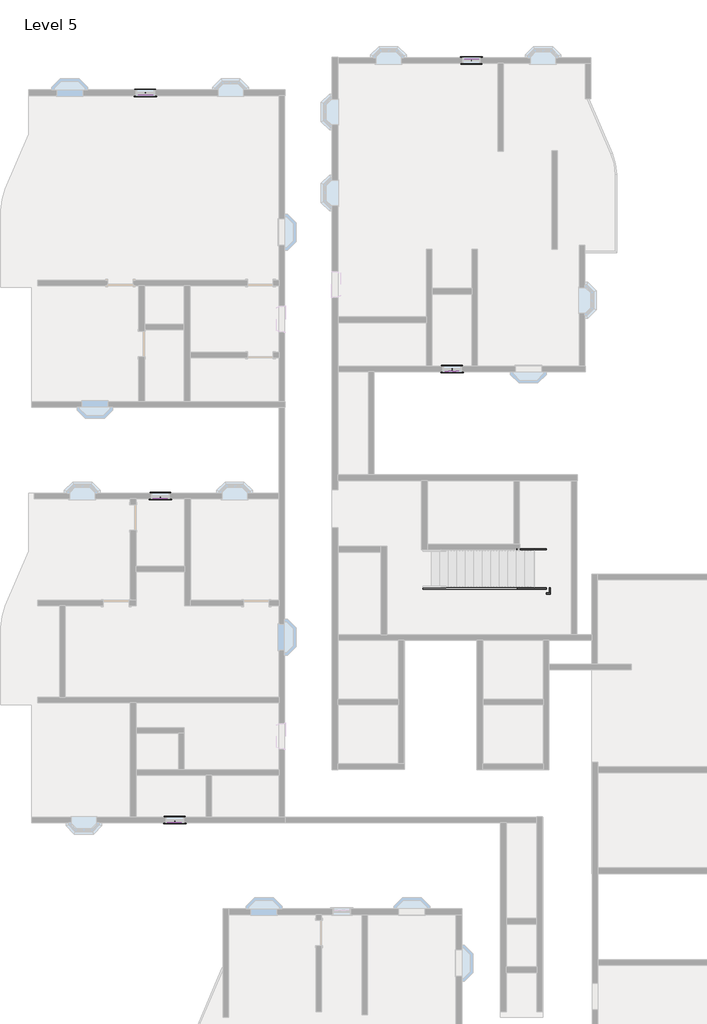
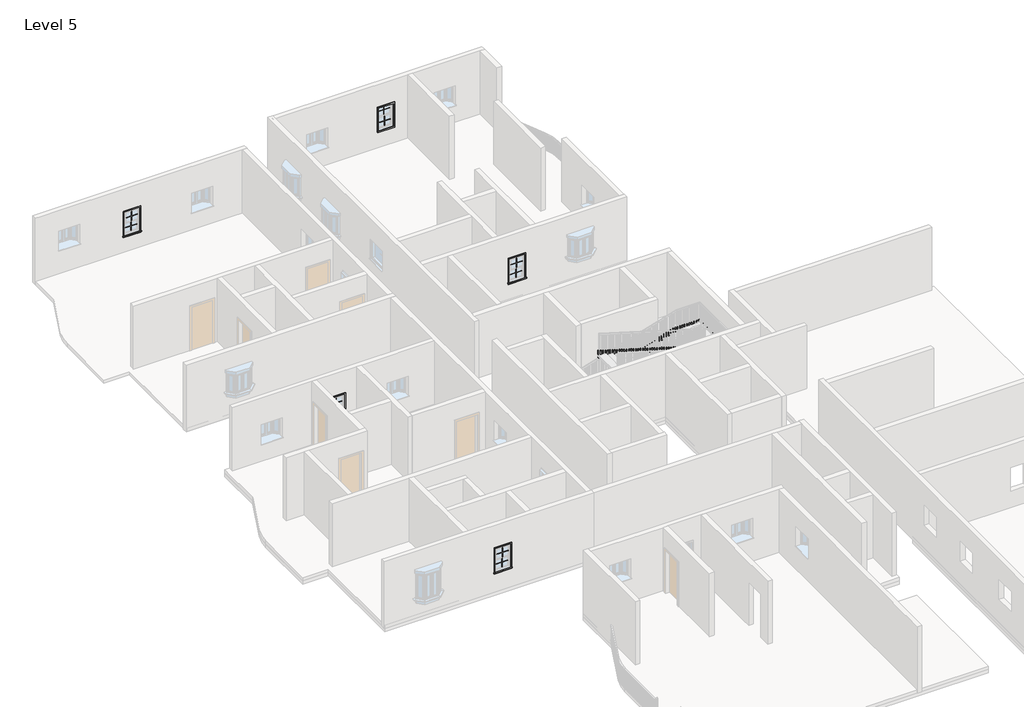
# One storey, part 14 of 14: 20 proxies, 6 members.
"""IFC4 building model written with IfcOpenShell, lengths in millimetres."""

from ifc_helpers import new_model, si_unit, frame, origin, place, context, project, spatial, polyline, outline, extrude, transform, mapped, element, save
from components import muntin_pattern_2x2_muntin_pattern_2x2_c35c595f, trim_window_exterior_flat_with_sill_e38017c9, trim_window_interior_flat_picture_frame_d728ed12

model = new_model("IFC4")

# Units and contexts
model_context = context("Model", 3, world=origin())
ifc_project = project(units=[si_unit("LENGTHUNIT", "METRE", prefix="MILLI")], contexts=[model_context])

# Site, building, storey
site = spatial("IfcSite", under=ifc_project)
building = spatial("IfcBuilding", under=site)
storey = spatial("IfcBuildingStorey", under=building, Name="Level 5", Elevation=12192.0)

# Proxies
placement = place(None, origin())
muntin_pattern_2x2_muntin_pattern_2x2_shape = muntin_pattern_2x2_muntin_pattern_2x2_c35c595f(model_context)
element("IfcBuildingElementProxy", 1, Name="Muntin Pattern_2x2 : Muntin Pattern_2x2", ObjectType="Muntin Pattern_2x2 : Muntin Pattern_2x2", at=placement, inside=storey, context=model_context, shape_type="MappedRepresentation", body=[
    mapped(muntin_pattern_2x2_muntin_pattern_2x2_shape, transform((-14639.3891351, 14368.0833494, 13662.025), x_axis=(-1.0, 0.0, 0.0), y_axis=(0.0, -1.0, 0.0), z_axis=(0.0, 0.0, 1.0))),
])
element("IfcBuildingElementProxy", 2, Name="Muntin Pattern_2x2 : Muntin Pattern_2x2", ObjectType="Muntin Pattern_2x2 : Muntin Pattern_2x2", at=placement, inside=storey, context=model_context, shape_type="MappedRepresentation", body=[
    mapped(muntin_pattern_2x2_muntin_pattern_2x2_shape, transform((-14639.3891351, 14412.5333494, 13182.6), x_axis=(-1.0, 0.0, 0.0), y_axis=(0.0, -1.0, 0.0), z_axis=(0.0, 0.0, 1.0))),
])
element("IfcBuildingElementProxy", 3, Name="Muntin Pattern_2x2 : Muntin Pattern_2x2", ObjectType="Muntin Pattern_2x2 : Muntin Pattern_2x2", at=placement, inside=storey, context=model_context, shape_type="MappedRepresentation", body=[
    mapped(muntin_pattern_2x2_muntin_pattern_2x2_shape, transform((-14125.0391351, 2785.6833494, 13662.025), x_axis=(-1.0, 0.0, 0.0), y_axis=(0.0, -1.0, 0.0), z_axis=(0.0, 0.0, 1.0))),
])
element("IfcBuildingElementProxy", 4, Name="Muntin Pattern_2x2 : Muntin Pattern_2x2", ObjectType="Muntin Pattern_2x2 : Muntin Pattern_2x2", at=placement, inside=storey, context=model_context, shape_type="MappedRepresentation", body=[
    mapped(muntin_pattern_2x2_muntin_pattern_2x2_shape, transform((-14125.0391351, 2830.1333494, 13182.6), x_axis=(-1.0, 0.0, 0.0), y_axis=(0.0, -1.0, 0.0), z_axis=(0.0, 0.0, 1.0))),
])
element("IfcBuildingElementProxy", 5, Name="Muntin Pattern_2x2 : Muntin Pattern_2x2", ObjectType="Muntin Pattern_2x2 : Muntin Pattern_2x2", at=placement, inside=storey, context=model_context, shape_type="MappedRepresentation", body=[
    mapped(muntin_pattern_2x2_muntin_pattern_2x2_shape, transform((-4206.3391351, 18910.0465905, 13662.025), x_axis=(-1.0, 0.0, 0.0), y_axis=(0.0, -1.0, 0.0), z_axis=(0.0, 0.0, 1.0))),
])
element("IfcBuildingElementProxy", 6, Name="Muntin Pattern_2x2 : Muntin Pattern_2x2", ObjectType="Muntin Pattern_2x2 : Muntin Pattern_2x2", at=placement, inside=storey, context=model_context, shape_type="MappedRepresentation", body=[
    mapped(muntin_pattern_2x2_muntin_pattern_2x2_shape, transform((-4206.3391351, 18954.4965905, 13182.6), x_axis=(-1.0, 0.0, 0.0), y_axis=(0.0, -1.0, 0.0), z_axis=(0.0, 0.0, 1.0))),
])
element("IfcBuildingElementProxy", 7, Name="Muntin Pattern_2x2 : Muntin Pattern_2x2", ObjectType="Muntin Pattern_2x2 : Muntin Pattern_2x2", at=placement, inside=storey, context=model_context, shape_type="MappedRepresentation", body=[
    mapped(muntin_pattern_2x2_muntin_pattern_2x2_shape, transform((-3514.1891351, 30066.9965905, 13662.025), x_axis=(1.0, 0.0, 0.0), y_axis=(0.0, 1.0, 0.0), z_axis=(0.0, 0.0, 1.0))),
])
element("IfcBuildingElementProxy", 8, Name="Muntin Pattern_2x2 : Muntin Pattern_2x2", ObjectType="Muntin Pattern_2x2 : Muntin Pattern_2x2", at=placement, inside=storey, context=model_context, shape_type="MappedRepresentation", body=[
    mapped(muntin_pattern_2x2_muntin_pattern_2x2_shape, transform((-3514.1891351, 30022.5465905, 13182.6), x_axis=(1.0, 0.0, 0.0), y_axis=(0.0, 1.0, 0.0), z_axis=(0.0, 0.0, 1.0))),
])
element("IfcBuildingElementProxy", 9, Name="Muntin Pattern_2x2 : Muntin Pattern_2x2", ObjectType="Muntin Pattern_2x2 : Muntin Pattern_2x2", at=placement, inside=storey, context=model_context, shape_type="MappedRepresentation", body=[
    mapped(muntin_pattern_2x2_muntin_pattern_2x2_shape, transform((-15175.9641351, 28782.5833494, 13662.025), x_axis=(-1.0, 0.0, 0.0), y_axis=(0.0, -1.0, 0.0), z_axis=(0.0, 0.0, 1.0))),
])
element("IfcBuildingElementProxy", 10, Name="Muntin Pattern_2x2 : Muntin Pattern_2x2", ObjectType="Muntin Pattern_2x2 : Muntin Pattern_2x2", at=placement, inside=storey, context=model_context, shape_type="MappedRepresentation", body=[
    mapped(muntin_pattern_2x2_muntin_pattern_2x2_shape, transform((-15175.9641351, 28827.0333494, 13182.6), x_axis=(-1.0, 0.0, 0.0), y_axis=(0.0, -1.0, 0.0), z_axis=(0.0, 0.0, 1.0))),
])
trim_window_exterior_flat_with_sill_shape = trim_window_exterior_flat_with_sill_e38017c9(model_context)
element("IfcBuildingElementProxy", 11, Name="Trim-Window-Exterior-Flat : with Sill", ObjectType="Trim-Window-Exterior-Flat : with Sill", at=placement, inside=storey, context=model_context, shape_type="MappedRepresentation", body=[
    mapped(trim_window_exterior_flat_with_sill_shape, transform((-14639.3891351, 14333.1583494, 14173.2), x_axis=(1.0, 0.0, 0.0), y_axis=(0.0, 0.0, 1.0), z_axis=(0.0, -1.0, 0.0))),
])
element("IfcBuildingElementProxy", 12, Name="Trim-Window-Exterior-Flat : with Sill", ObjectType="Trim-Window-Exterior-Flat : with Sill", at=placement, inside=storey, context=model_context, shape_type="MappedRepresentation", body=[
    mapped(trim_window_exterior_flat_with_sill_shape, transform((-14125.0391351, 2750.7583494, 14173.2), x_axis=(1.0, 0.0, 0.0), y_axis=(0.0, 0.0, 1.0), z_axis=(0.0, -1.0, 0.0))),
])
element("IfcBuildingElementProxy", 13, Name="Trim-Window-Exterior-Flat : with Sill", ObjectType="Trim-Window-Exterior-Flat : with Sill", at=placement, inside=storey, context=model_context, shape_type="MappedRepresentation", body=[
    mapped(trim_window_exterior_flat_with_sill_shape, transform((-4206.3391351, 18875.1215905, 14173.2), x_axis=(1.0, 0.0, 0.0), y_axis=(0.0, 0.0, 1.0), z_axis=(0.0, -1.0, 0.0))),
])
element("IfcBuildingElementProxy", 14, Name="Trim-Window-Exterior-Flat : with Sill", ObjectType="Trim-Window-Exterior-Flat : with Sill", at=placement, inside=storey, context=model_context, shape_type="MappedRepresentation", body=[
    mapped(trim_window_exterior_flat_with_sill_shape, transform((-3514.1891351, 30101.9215905, 14173.2), x_axis=(-1.0, 0.0, 0.0), y_axis=(0.0, 0.0, 1.0), z_axis=(0.0, 1.0, 0.0))),
])
element("IfcBuildingElementProxy", 15, Name="Trim-Window-Exterior-Flat : with Sill", ObjectType="Trim-Window-Exterior-Flat : with Sill", at=placement, inside=storey, context=model_context, shape_type="MappedRepresentation", body=[
    mapped(trim_window_exterior_flat_with_sill_shape, transform((-15175.9641351, 28747.6583494, 14173.2), x_axis=(1.0, 0.0, 0.0), y_axis=(0.0, 0.0, 1.0), z_axis=(0.0, -1.0, 0.0))),
])
trim_window_interior_flat_picture_frame_shape = trim_window_interior_flat_picture_frame_d728ed12(model_context)
element("IfcBuildingElementProxy", 16, Name="Trim-Window-Interior-Flat : Picture Frame", ObjectType="Trim-Window-Interior-Flat : Picture Frame", at=placement, inside=storey, context=model_context, shape_type="MappedRepresentation", body=[
    mapped(trim_window_interior_flat_picture_frame_shape, transform((-14639.3891351, 14536.3583494, 14173.2), x_axis=(-1.0, 0.0, 0.0), y_axis=(0.0, 0.0, 1.0), z_axis=(0.0, 1.0, 0.0))),
])
element("IfcBuildingElementProxy", 17, Name="Trim-Window-Interior-Flat : Picture Frame", ObjectType="Trim-Window-Interior-Flat : Picture Frame", at=placement, inside=storey, context=model_context, shape_type="MappedRepresentation", body=[
    mapped(trim_window_interior_flat_picture_frame_shape, transform((-14125.0391351, 2953.9583494, 14173.2), x_axis=(-1.0, 0.0, 0.0), y_axis=(0.0, 0.0, 1.0), z_axis=(0.0, 1.0, 0.0))),
])
element("IfcBuildingElementProxy", 18, Name="Trim-Window-Interior-Flat : Picture Frame", ObjectType="Trim-Window-Interior-Flat : Picture Frame", at=placement, inside=storey, context=model_context, shape_type="MappedRepresentation", body=[
    mapped(trim_window_interior_flat_picture_frame_shape, transform((-4206.3391351, 19078.3215905, 14173.2), x_axis=(-1.0, 0.0, 0.0), y_axis=(0.0, 0.0, 1.0), z_axis=(0.0, 1.0, 0.0))),
])
element("IfcBuildingElementProxy", 19, Name="Trim-Window-Interior-Flat : Picture Frame", ObjectType="Trim-Window-Interior-Flat : Picture Frame", at=placement, inside=storey, context=model_context, shape_type="MappedRepresentation", body=[
    mapped(trim_window_interior_flat_picture_frame_shape, transform((-3514.1891351, 29898.7215905, 14173.2), x_axis=(1.0, 0.0, 0.0), y_axis=(0.0, 0.0, 1.0), z_axis=(0.0, -1.0, 0.0))),
])
element("IfcBuildingElementProxy", 20, Name="Trim-Window-Interior-Flat : Picture Frame", ObjectType="Trim-Window-Interior-Flat : Picture Frame", at=placement, inside=storey, context=model_context, shape_type="MappedRepresentation", body=[
    mapped(trim_window_interior_flat_picture_frame_shape, transform((-15175.9641351, 28950.8583494, 14173.2), x_axis=(-1.0, 0.0, 0.0), y_axis=(0.0, 0.0, 1.0), z_axis=(0.0, 1.0, 0.0))),
])

# Members
element("IfcMember", 21, ObjectType="Stringer - 2\" Width", at=placement, inside=storey, context=model_context, shape_type="SweptSolid", body=[
    extrude(outline(polyline([(12383.5995961, -5254.0891351), (12192.0, -5254.0891351), (12192.0, -4832.019314), (13639.8, -6.019314), (13639.8, -1066.7544553), (12383.5995961, -5254.0891351)])), frame((0.0, 12506.0715905, 0.0), z_axis=(0.0, 1.0, 0.0), x_axis=(0.0, 0.0, 1.0)), (0.0, 0.0, 1.0), 50.8),
])
element("IfcMember", 22, ObjectType="Stringer - 2\" Width", at=placement, inside=storey, context=model_context, shape_type="SweptSolid", body=[
    extrude(outline(polyline([(54.5108649, 12556.8715905), (105.3108649, 12556.8715905), (105.3108649, 9478.4949943), (54.5108649, 9478.4949943), (54.5108649, 12556.8715905)])), frame((0.0, 0.0, 13335.0), z_axis=(0.0, 0.0, 1.0), x_axis=(1.0, 0.0, 0.0)), (0.0, 0.0, 1.0), 304.8),
])
element("IfcMember", 23, ObjectType="Stringer - 2\" Width", at=placement, inside=storey, context=model_context, shape_type="SweptSolid", body=[
    extrude(outline(polyline([(13335.0, 105.3108649), (13427.5395961, 105.3108649), (15035.3595961, -5254.0891351), (14717.1390537, -5254.0891351), (13335.0, -646.9589562), (13335.0, 105.3108649)])), frame((0.0, 9427.6949943, 0.0), z_axis=(0.0, 1.0, 0.0), x_axis=(0.0, 0.0, 1.0)), (0.0, 0.0, 1.0), 50.8),
])
element("IfcMember", 24, ObjectType="Stringer - 2\" Width", at=placement, inside=storey, context=model_context, shape_type="SweptSolid", body=[
    extrude(outline(polyline([(12383.5995961, -5254.0891351), (12192.0, -5254.0891351), (12192.0, -4832.019314), (13421.7390537, -732.8891351), (13639.8, -732.8891351), (13639.8, -1066.7544553), (12383.5995961, -5254.0891351)])), frame((0.0, 11103.4082924, 0.0), z_axis=(0.0, 1.0, 0.0), x_axis=(0.0, 0.0, 1.0)), (0.0, 0.0, 1.0), 50.8),
])
element("IfcMember", 25, ObjectType="Stringer - 2\" Width", at=placement, inside=storey, context=model_context, shape_type="SweptSolid", body=[
    extrude(outline(polyline([(-732.8891351, 11154.2082924), (-682.0891351, 11154.2082924), (-682.0891351, 10976.4082924), (-732.8891351, 10976.4082924), (-732.8891351, 11154.2082924)])), frame((0.0, 0.0, 13335.0), z_axis=(0.0, 0.0, 1.0), x_axis=(1.0, 0.0, 0.0)), (0.0, 0.0, 1.0), 304.8),
])
element("IfcMember", 26, ObjectType="Stringer - 2\" Width", at=placement, inside=storey, context=model_context, shape_type="SweptSolid", body=[
    extrude(outline(polyline([(13345.5390537, -682.0891351), (13663.7595961, -682.0891351), (15035.3595961, -5254.0891351), (14717.1390537, -5254.0891351), (13345.5390537, -682.0891351)])), frame((0.0, 10925.6082924, 0.0), z_axis=(0.0, 1.0, 0.0), x_axis=(0.0, 0.0, 1.0)), (0.0, 0.0, 1.0), 50.8),
])

save(model, "model.ifc")

# Revit data of these elements
# Type "Muntin Pattern_2x2 : Muntin Pattern_2x2"
#   Width [instance default] = 4' - 0"
#   Thickness = 0' - 0 1/2"
#   Height [instance default] = 4' - 0"
#   Distance = 0' - 0 3/4"
#   Interior Material [instance default] = none
#   Exterior Material [instance default] = none
#   Default Elevation = 0
# Type "Trim-Window-Exterior-Flat : with Sill"
#   Trim Width = 0' - 2 1/4"
#   Trim Thickness_Picture Frame = 0' - 1 1/4"
#   Trim Thickness_with Sill = 0' - 0 3/4"
#   Sill Thickness = 0' - 1 1/4"
#   Opening Width [instance default] = 2' - 0"
#   Opening Height [instance default] = 3' - 0"
#   Default Elevation = 4' - 0"
#   Sill = yes
#   Picture Frame = no
#   Trim Material [instance default] = none
# Type "Trim-Window-Interior-Flat : Picture Frame"
#   Trim Thickness_Picture Frame = 0' - 1 1/4"
#   Trim Width = 0' - 2 1/4"
#   Trim Thickness_with Sill = 0' - 0 3/4"
#   Sill Thickness = 0' - 1 1/4"
#   Opening Width [instance default] = 2' - 0"
#   Opening Height [instance default] = 3' - 0"
#   Default Elevation = 4' - 0"
#   Sill = no
#   Picture Frame = yes
#   Trim Material [instance default] = none
# Elements 1, 2, 3, 4, 5, 6, 7, 8, 9, 10 (IfcBuildingElementProxy, "Muntin Pattern_2x2 : Muntin Pattern_2x2")
#   Width = 1' - 8"
#   Height = 1' - 5 1/8"
#   Interior Material = Wood - Stained
#   Exterior Material = Clad - White
#   Phase Created = New Construction
#   Materials on its faces: "Clad - White", "Wood - Stained"
# Elements 11, 12, 13, 14, 15 (IfcBuildingElementProxy, "Trim-Window-Exterior-Flat : with Sill")
#   Opening Width = 2' - 2"
#   Opening Height = 3' - 6"
#   Trim Material = Clad - White
#   Phase Created = New Construction
#   Materials on its faces: "Clad - White"
# Elements 16, 17, 18, 19, 20 (IfcBuildingElementProxy, "Trim-Window-Interior-Flat : Picture Frame")
#   Opening Width = 2' - 2"
#   Opening Height = 3' - 6"
#   Trim Material = Wood - Stained
#   Phase Created = New Construction
#   Materials on its faces: "Wood - Stained"
# Elements 21, 22, 23, 24, 25, 26 (IfcMember, "Stringer - 2\" Width")
#   Phase Created = New Construction
# Materials
#   "Clad - White": class "Wood", colour RGB 242 242 238, transparency 0, Cost = 0
#   "Wood - Stained": class "Wood", colour RGB 224 178 126, transparency 0, Cost = 0
